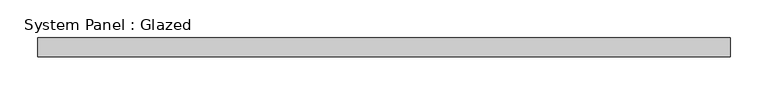
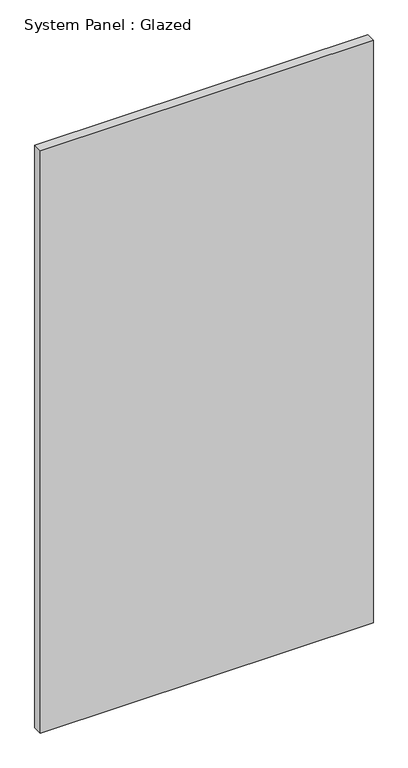
"""IFC4 building model written with IfcOpenShell, lengths in millimetres: plate geometry, System Panel : Glazed."""

from ifc_helpers import new_model, si_unit, origin, origin_with_axes, place, context, project, spatial, polyline, outline, extrude, source, transform, mapped, element, save


def system_panel_glazed_2247c2a6(model_context):
    return source(origin(), model_context, "Body", "SweptSolid", [
        extrude(outline(polyline([(460.4808778, 19.05), (-460.4808778, 19.05), (-460.4808778, 44.45), (460.4808778, 44.45), (460.4808778, 19.05)])), origin_with_axes(), (0.0, 0.0, 1.0), 1701.8),
    ])


if __name__ == "__main__":
    model = new_model("IFC4")
    model_context = context("Model", 3, world=origin())
    ifc_project = project(units=[si_unit("LENGTHUNIT", "METRE", prefix="MILLI")], contexts=[model_context])
    site = spatial("IfcSite", under=ifc_project)
    building = spatial("IfcBuilding", under=site)
    placement = place(None, origin())
    system_panel_glazed_shape = system_panel_glazed_2247c2a6(model_context)
    element("IfcPlate", 1, ObjectType="System Panel : Glazed", at=placement, inside=building, context=model_context, shape_type="MappedRepresentation", body=[
        mapped(system_panel_glazed_shape, transform((0.0, 0.0, 0.0), x_axis=(1.0, 0.0, 0.0), y_axis=(0.0, 1.0, 0.0), z_axis=(0.0, 0.0, 1.0))),
    ])
    save(model, "model.ifc")

# Revit data of these elements
# Type "System Panel : Glazed"
#   Construction Type Id = "GSP4R"
#   Analytic Construction = "1/8 in Pilkington single glazing"
#   Visual Light Transmittance = 0.9
#   Solar Heat Gain Coefficient = 0.86
#   Heat Transfer Coefficient (U) = 1.18115 BTU/(h·ft²·°F)
#   Define Thermal Properties by = 1
# Element 1 (IfcPlate, "System Panel : Glazed")
#   Materials on its faces: "Glass"
# Materials
#   "Glass": class "Glass", colour RGB 154 182 205, transparency 0.85, Description = "Soda Lime Glass", Cost = 0
